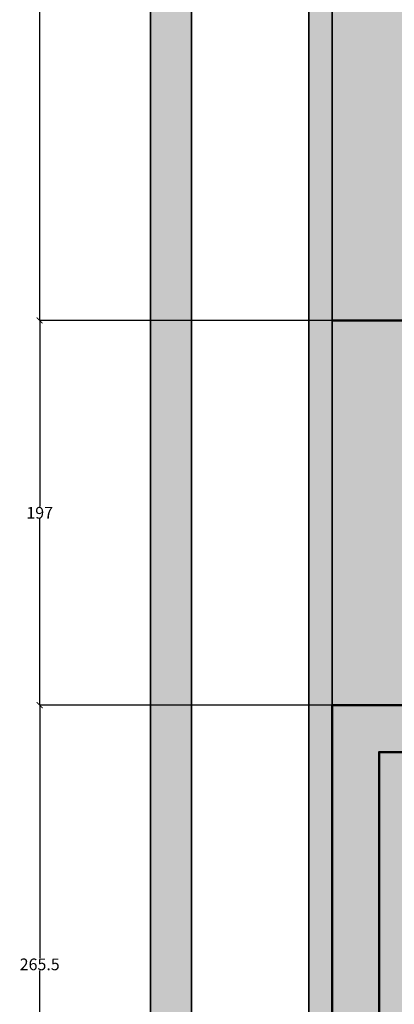
# Model space of a CAD drawing. Units: inches. Extents: x 925 to 2834, y 111 to 1355.
# Tile 2 of 25: x 925 to 1116, y 377 to 882. Entities that reach past the tile are written whole.
import ezdxf

# ---------------------------------------------------------------- set-up
doc = ezdxf.new("R2010")
doc.units = ezdxf.units.IN
doc.header["$MEASUREMENT"] = 0
for name, color, linetype, lineweight in [('A-ANNO-DIMS', 2, 'Continuous', 18), ('A-ANNO-TTLB', 7, 'Continuous', 35), ('A-FLOR-PATT', 252, 'Continuous', 13), ('A-WALL', 7, 'Continuous', 50)]:
    doc.layers.add(name, color=color, linetype=linetype, lineweight=lineweight)
doc.styles.get("Standard").update_dxf_attribs({"font": 'arial.ttf'})
doc.dimstyles.get("Standard").update_dxf_attribs({"dimtxt": 6, "dimasz": 3, "dimexe": 0.18, "dimexo": 0.0625, "dimgap": 0.09, "dimtad": 0, "dimtih": 1, "dimtoh": 1, "dimdec": 1, "dimzin": 0, "dimdsep": 46, "dimlunit": 3, "dimtxsty": 'Standard', "dimblk": 'ARCHTICK', "dimcen": 0.09, "dimadec": 0, "dimazin": 0, "dimtfac": 1, "dimtdec": 1, "dimtofl": 0, "dimtmove": 0, "dimatfit": 3, "dimfxl": 1, "dimtolj": 1, "dimtzin": 0, "dimarcsym": 0})

# ---------------------------------------------------------------- blocks, each defined once
blk = doc.blocks.new('_ArchTick')
at = {"color": 0, "linetype": 'ByBlock', "const_width": 0.15}
blk.add_lwpolyline([(-0.5, -0.5), (0.5, 0.5)], dxfattribs=at)
blk = doc.blocks.new('*D25')
at = {"layer": 'A-ANNO-DIMS', "color": 0, "lineweight": -2, "transparency": 16777216}
for p, q in [((1200.21, 727.53), (1200.21, 115.18)), ((1084.71, 265.03), (1084.71, 115.18)), ((1084.71, 115.36), (1132.51, 115.36)), ((1200.21, 115.36), (1152.42, 115.36))]:
    blk.add_line(p, q, dxfattribs=at)
at = {"layer": 'Defpoints', "color": 0, "transparency": 16777216}
for p in [(1200.21, 727.59), (1084.71, 265.09), (1200.21, 115.36)]:
    blk.add_point(p, dxfattribs=at)
at = {"layer": 'A-ANNO-DIMS', "color": 0, "lineweight": -2, "transparency": 16777216, "xscale": 3, "yscale": 3, "zscale": 3, "rotation": 180}
blk.add_blockref('_ArchTick', (1084.71, 115.36), dxfattribs=at)
at = {"layer": 'A-ANNO-DIMS', "color": 0, "lineweight": -2, "transparency": 16777216, "xscale": 3, "yscale": 3, "zscale": 3}
blk.add_blockref('_ArchTick', (1200.21, 115.36), dxfattribs=at)
at = {"layer": 'A-ANNO-DIMS', "color": 0, "transparency": 16777216, "insert": (1142.46, 115.36), "char_height": 6, "attachment_point": 5}
blk.add_mtext('\\A1;115.5', dxfattribs=at)
blk = doc.blocks.new('*D34')
at = {"layer": 'A-ANNO-DIMS', "color": 0, "lineweight": -2, "transparency": 16777216}
for p, q in [((1084.65, 530.59), (934.81, 530.59)), ((934.99, 530.59), (934.99, 400.99)), ((934.99, 265.09), (934.99, 394.69)), ((1084.65, 265.09), (934.81, 265.09))]:
    blk.add_line(p, q, dxfattribs=at)
at = {"layer": 'Defpoints', "color": 0, "transparency": 16777216}
for p in [(934.99, 530.59), (1084.71, 530.59), (1084.71, 265.09)]:
    blk.add_point(p, dxfattribs=at)
at = {"layer": 'A-ANNO-DIMS', "color": 0, "lineweight": -2, "transparency": 16777216, "xscale": 3, "yscale": 3, "zscale": 3}
for p, rotation in [((934.99, 530.59), 90), ((934.99, 265.09), 270)]:
    blk.add_blockref('_ArchTick', p, dxfattribs=dict(at, rotation=rotation))
at = {"layer": 'A-ANNO-DIMS', "color": 0, "transparency": 16777216, "insert": (934.99, 397.84), "char_height": 6, "attachment_point": 5}
blk.add_mtext('\\A1;265.5', dxfattribs=at)
blk = doc.blocks.new('*D35')
at = {"layer": 'A-ANNO-DIMS', "color": 0, "lineweight": -2, "transparency": 16777216}
for p, q in [((1084.65, 727.59), (934.81, 727.59)), ((934.99, 727.59), (934.99, 632.24)), ((934.99, 530.59), (934.99, 625.94)), ((1084.65, 530.59), (934.81, 530.59))]:
    blk.add_line(p, q, dxfattribs=at)
at = {"layer": 'Defpoints', "color": 0, "transparency": 16777216}
for p in [(934.99, 727.59), (1084.71, 727.59), (1084.71, 530.59)]:
    blk.add_point(p, dxfattribs=at)
at = {"layer": 'A-ANNO-DIMS', "color": 0, "lineweight": -2, "transparency": 16777216, "xscale": 3, "yscale": 3, "zscale": 3}
for p, rotation in [((934.99, 727.59), 90), ((934.99, 530.59), 270)]:
    blk.add_blockref('_ArchTick', p, dxfattribs=dict(at, rotation=rotation))
at = {"layer": 'A-ANNO-DIMS', "color": 0, "transparency": 16777216, "insert": (934.99, 629.09), "char_height": 6, "attachment_point": 5}
blk.add_mtext('\\A1;197', dxfattribs=at)
blk = doc.blocks.new('*D36')
at = {"layer": 'A-ANNO-DIMS', "color": 0, "lineweight": -2, "transparency": 16777216}
for p, q in [((1084.65, 1081.59), (934.81, 1081.59)), ((934.99, 1081.59), (934.99, 907.74)), ((934.99, 727.59), (934.99, 901.43)), ((1084.65, 727.59), (934.81, 727.59))]:
    blk.add_line(p, q, dxfattribs=at)
at = {"layer": 'Defpoints', "color": 0, "transparency": 16777216}
for p in [(934.99, 1081.59), (1084.71, 1081.59), (1084.71, 727.59)]:
    blk.add_point(p, dxfattribs=at)
at = {"layer": 'A-ANNO-DIMS', "color": 0, "lineweight": -2, "transparency": 16777216, "xscale": 3, "yscale": 3, "zscale": 3}
for p, rotation in [((934.99, 1081.59), 90), ((934.99, 727.59), 270)]:
    blk.add_blockref('_ArchTick', p, dxfattribs=dict(at, rotation=rotation))
at = {"layer": 'A-ANNO-DIMS', "color": 0, "transparency": 16777216, "insert": (934.99, 904.59), "char_height": 6, "attachment_point": 5}
blk.add_mtext('\\A1;354', dxfattribs=at)

msp = doc.modelspace()

# ---------------------------------------------------------------- hatches: boundary and pattern name
at = {"layer": 'A-FLOR-PATT', "transparency": 33554605}
h = msp.add_hatch(color=256, dxfattribs=at)
h.dxf.hatch_style = 1
h.paths.add_polyline_path([(1931.688, 1294.5638), (991.7375, 1294.5638), (991.7375, 172.1134), (1931.688, 172.1134)])
h.paths.add_polyline_path([(1910.7128, 1273.5886), (1910.7128, 193.0886), (1012.7128, 193.0886), (1012.7128, 1273.5886)], flags=16)
h.paths.add_polyline_path([(1850.7128, 1213.5886), (1850.7128, 253.0886), (1072.7128, 253.0886), (1072.7128, 1213.5886)], flags=0)
h.paths.add_polyline_path([(1838.7128, 1201.5886), (1838.7128, 265.0886), (1084.7128, 265.0886), (1084.7128, 530.5886), (1084.7128, 1201.5886)], flags=0)
h.paths.add_polyline_path([(1547.6758, 1155.7396), (1547.6758, 1119.115), (1513.0687, 1119.115), (1513.0687, 1155.7396)], flags=0)
h.paths.add_polyline_path([(1600.1067, 1154.9439), (1634.7139, 1154.9439), (1634.7139, 1119.115), (1600.1067, 1119.115)], flags=0)
h.paths.add_polyline_path([(1505.2502, 1144.5358), (1505.2502, 1119.115), (1470.643, 1119.115), (1470.643, 1144.5358)], flags=0)
h.paths.add_polyline_path([(1559.1357, 1141.0962), (1593.7428, 1141.0962), (1593.7428, 1119.115), (1559.1357, 1119.115)], flags=0)
h.paths.add_polyline_path([(1462.8966, 1154.9439), (1462.8966, 1119.115), (1428.2895, 1119.115), (1428.2895, 1154.9439)], flags=0)
h.paths.add_polyline_path([(1642.4603, 1144.5358), (1677.0675, 1144.5358), (1677.0675, 1119.115), (1642.4603, 1119.115)], flags=0)
h.paths.add_polyline_path([(1422.3508, 1141.0962), (1422.3508, 1119.115), (1387.7436, 1119.115), (1387.7436, 1141.0962)], flags=0)
h.paths.add_polyline_path([(1684.8859, 1155.7396), (1719.4931, 1155.7396), (1719.4931, 1119.115), (1684.8859, 1119.115)], flags=0)
h.paths.add_polyline_path([(1718.7128, 1081.5886), (1718.7128, 1050.1249), (1715.7128, 1050.1249), (1715.7128, 1026.1249), (1715.7128, 1002.1249), (1718.7128, 1002.1249), (1730.7128, 1002.1249), (1730.7128, 998.1249), (1730.7128, 990.1249), (1730.7128, 986.1249), (1718.7128, 986.1249), (1718.7128, 893.5886), (1715.3735, 893.5886), (1715.3735, 891.5886), (1713.3735, 891.5886, 0.41421356), (1677.3735, 855.5886), (1713.3735, 855.5886), (1713.3735, 853.5886), (1715.3735, 853.5886), (1715.3735, 851.5886), (1718.7128, 851.5886), (1718.7128, 821.5865), (1734.4655, 821.5865), (1734.3735, 819.5886, -0.41421356), (1712.4415, 793.5886), (1712.4415, 791.5886), (1718.7128, 791.5886), (1718.7128, 717.5886), (1718.7128, 669.5886), (1732.7128, 669.5886), (1732.7128, 665.5886), (1732.7128, 641.5886), (1732.7128, 634.5886), (1732.7128, 610.5886), (1732.7128, 603.5886), (1718.7128, 603.5886), (1718.7128, 385.0886), (1434.2128, 385.0886), (1434.2128, 530.5886), (1410.2128, 530.5886), (1408.2128, 530.5886), (1408.2128, 532.5886, 0.41421356), (1372.2128, 568.5886), (1372.2128, 532.5886), (1370.2128, 532.5886), (1370.2128, 530.5886), (1368.2128, 530.5886), (1282.2128, 530.5886), (1210.2128, 530.5886), (1200.2128, 530.5886), (1200.2128, 542.1915), (1183.2307, 542.1915), (1183.2307, 546.1915), (1200.2128, 546.1915), (1200.2128, 572.1915), (1183.2307, 572.1915), (1183.2307, 576.1915), (1200.2128, 576.1915), (1200.2128, 727.5886), (1210.2128, 727.5886), (1234.2128, 727.5886), (1259.7128, 727.5886), (1259.7128, 775.5886), (1259.7128, 799.5886), (1259.7128, 847.5886), (1259.7128, 993.5872), (1259.7128, 1065.5872), (1259.7128, 1071.5886), (1219.6318, 1071.5886), (1219.6318, 1081.5886), (1084.7128, 1081.5886), (1084.7128, 1119.115), (1256.8974, 1119.115), (1256.8974, 1154.9439), (1291.5046, 1154.9439), (1291.5046, 1119.115), (1256.8974, 1119.115), (1256.6723, 1081.5886), (1293.7128, 1081.5886), (1341.7128, 1081.5886), (1341.7128, 1093.5886), (1347.7128, 1093.5886), (1371.7128, 1093.5886), (1377.7128, 1093.5886), (1377.7128, 1081.5886), (1668.7128, 1081.5886), (1668.7128, 1117.5886), (1675.7128, 1117.5886), (1711.7128, 1117.5886), (1718.7128, 1117.5886)], flags=0)
h.paths.add_polyline_path([(1376.2838, 1155.7396), (1376.2838, 1119.115), (1341.6766, 1119.115), (1341.6766, 1155.7396)], flags=0)
h.paths.add_polyline_path([(1341.7128, 1076.0886), (1293.7128, 1076.0886), (1293.7128, 1071.5886), (1269.7128, 1071.5886), (1269.7128, 1065.5872), (1266.7128, 1065.5872), (1266.7128, 1029.5872), (1265.7128, 1029.5872), (1265.7128, 993.5872), (1269.7128, 993.5872), (1269.7128, 903.5886), (1269.7128, 893.5886), (1269.7128, 847.5886), (1265.2128, 847.5886), (1265.2128, 799.5886), (1269.7128, 799.5886), (1269.7128, 775.5886), (1265.2128, 775.5886), (1265.2128, 727.5886), (1269.7128, 727.5886), (1444.2128, 727.5886), (1444.2128, 717.5886), (1234.2128, 717.5886), (1234.2128, 722.0886), (1210.2128, 722.0886), (1210.2128, 717.5886), (1210.2128, 540.5886), (1210.2128, 536.0886), (1282.2128, 536.0886), (1282.2128, 535.0886), (1210.2128, 535.0886), (1210.2128, 540.5886), (1210.2128, 717.5886), (1210.2128, 723.0886), (1234.2128, 723.0886), (1234.2128, 717.5886), (1444.2128, 717.5886), (1444.2128, 727.5886), (1269.7128, 727.5886), (1264.2128, 727.5886), (1264.2128, 775.5886), (1269.7128, 775.5886), (1269.7128, 799.5886), (1264.2128, 799.5886), (1264.2128, 847.5886), (1269.7128, 847.5886), (1269.7128, 893.5886), (1269.7128, 903.5886), (1269.7128, 993.5872), (1264.7128, 993.5872), (1264.7128, 1029.5872), (1265.7128, 1029.5872), (1265.7128, 1065.5872), (1269.7128, 1065.5872), (1269.7128, 1071.5886), (1293.7128, 1071.5886), (1293.7128, 1077.0886), (1341.7128, 1077.0886)], flags=0)
h.paths.add_polyline_path([(1730.9529, 1141.0962), (1765.5601, 1141.0962), (1765.5601, 1119.115), (1730.9529, 1119.115)], flags=0)
h.paths.add_polyline_path([(1333.8582, 1144.5358), (1333.8582, 1119.115), (1299.251, 1119.115), (1299.251, 1144.5358)], flags=0)
h.paths.add_polyline_path([(1592.7128, 968.5886), (1596.0342, 968.5886), (1602.7128, 968.5886), (1708.7128, 968.5886), (1708.7128, 903.5886), (1602.7128, 903.5886), (1602.7128, 938.5886), (1592.7128, 938.5886), (1592.7128, 903.5886), (1451.7128, 903.5886), (1451.7128, 893.5886), (1511.7128, 893.5886), (1511.7128, 881.5886), (1515.2128, 881.5886), (1518.7128, 881.5886), (1518.7128, 893.5886), (1592.7128, 893.5886), (1592.7128, 799.5886), (1518.7128, 799.5886), (1518.7128, 857.5886), (1511.7128, 857.5886), (1511.7128, 799.5886), (1511.7128, 772.0886), (1521.7128, 772.0886), (1521.7128, 792.5886), (1592.7128, 792.5886), (1592.7128, 727.5886), (1521.7128, 727.5886), (1521.7128, 748.0886), (1511.7128, 748.0886), (1511.7128, 717.5886), (1708.7128, 717.5886), (1714.2128, 717.5886), (1714.2128, 669.5886), (1708.7128, 669.5886), (1708.7128, 641.5886), (1492.2128, 641.5886), (1492.2128, 631.5886), (1621.2128, 631.5886), (1621.2128, 443.0886), (1625.7128, 443.0886), (1625.7128, 503.0886), (1625.7128, 507.5886), (1625.7128, 631.5886), (1708.7128, 631.5886), (1708.7128, 507.5886), (1655.7128, 507.5886), (1655.7128, 503.0886), (1708.7128, 503.0886), (1708.7128, 395.0886), (1625.7128, 395.0886), (1625.7128, 419.0886), (1621.2128, 419.0886), (1621.2128, 395.0886), (1482.2128, 395.0886), (1482.2128, 385.0886), (1434.2128, 385.0886), (1434.2128, 433.0886), (1444.2128, 433.0886), (1444.2128, 631.5886), (1450.2128, 631.5886), (1450.2128, 634.91), (1452.2128, 634.91), (1452.2128, 669.5886), (1454.2128, 669.5886, -0.40021217), (1490.1712, 635.3173), (1492.2128, 635.3173), (1492.2128, 641.5886), (1564.7128, 641.5886), (1564.7128, 677.5886), (1672.7128, 677.5886), (1672.7128, 681.5886), (1564.7128, 681.5886), (1564.7128, 717.5886), (1511.7128, 717.5886), (1511.7128, 748.0886), (1511.7128, 772.0886), (1511.7128, 799.5886), (1511.7128, 857.5886), (1511.8913, 857.5886), (1511.8913, 859.5886), (1515.6201, 859.5886, 0.41421356), (1537.552, 879.5886), (1513.552, 879.5886), (1511.8913, 879.5886), (1511.8913, 881.5886), (1511.7128, 881.5886), (1511.7128, 893.5886), (1451.7128, 893.5886), (1451.7128, 903.5886), (1592.7128, 903.5886), (1592.7128, 938.5886), (1592.7128, 940.5886), (1596.4415, 940.5886, 0.41421356), (1618.3735, 966.5886), (1594.3735, 966.5886), (1592.7128, 966.5886)], flags=0)
h.paths.add_polyline_path([(1377.7128, 903.5886), (1377.7128, 893.5886), (1305.7128, 893.5886), (1305.7128, 903.5886)], flags=0)
h.paths.add_polyline_path([(1708.7128, 821.5886), (1712.0342, 821.5886), (1712.0342, 819.5886), (1710.3735, 819.5886), (1708.7128, 819.5886)], flags=0)
h.paths.add_polyline_path([(1576.7128, 695.1992), (1575.5896, 693.6649), (1575.9687, 694.6994), (1575.4438, 695.1992), (1575.9687, 695.699), (1575.5896, 696.7335)], flags=0)
h.paths.add_polyline_path([(1565.9817, 662.3134), (1565.4568, 661.8136), (1565.8359, 660.7791), (1564.7128, 662.3134), (1565.8359, 663.8477), (1565.4568, 662.8132)], flags=0)
h.paths.add_polyline_path([(1444.2128, 433.0886), (1444.2128, 395.0886), (1482.2128, 395.0886), (1482.2128, 389.0886), (1438.2128, 389.0886), (1438.2128, 391.8608), (1438.2128, 433.0886)], flags=0)
h.paths.add_polyline_path([(1410.2128, 506.5886), (1410.2128, 289.0886), (1108.7128, 289.0886), (1108.7128, 506.5886)], flags=0)
h.paths.add_polyline_path([(1612.3153, 838.3016), (1680.4151, 838.3016), (1680.4151, 851.3131), (1612.3153, 851.3131)], flags=8)
h.paths.add_polyline_path([(1208.3174, 395.0436), (1282.1017, 395.0436), (1282.1017, 408.0552), (1208.3174, 408.0552)], flags=8)
h.paths.add_polyline_path([(1291.8049, 598.7427), (1369.8017, 598.7427), (1369.8017, 611.7542), (1291.8049, 611.7542)], flags=8)
h.paths.add_polyline_path([(1119.679, 917.3022), (1191.0817, 917.3022), (1191.0817, 930.3137), (1119.679, 930.3137)], flags=8)
h.paths.add_polyline_path([(1332.2261, 815.9808), (1410.2258, 815.9808), (1410.2258, 829.001), (1332.2261, 829.001)], flags=8)
h.paths.add_polyline_path([(1390.9013, 955.8158), (1475.4981, 955.8158), (1475.4981, 968.8273), (1390.9013, 968.8273)], flags=8)
h.paths.add_polyline_path([(1620.3436, 998.9325), (1688.4434, 998.9325), (1688.4434, 1011.944), (1620.3436, 1011.944)], flags=8)
h.paths.add_polyline_path([(1620.3436, 914.1039), (1691.7405, 914.1039), (1691.7405, 927.1155), (1620.3436, 927.1155)], flags=8)
h.paths.add_polyline_path([(1521.4542, 816.005), (1589.5569, 816.005), (1589.5569, 829.0253), (1521.4542, 829.0253)], flags=8)
h.paths.add_polyline_path([(1528.524, 740.3497), (1602.3082, 740.3497), (1602.3082, 753.3613), (1528.524, 753.3613)], flags=8)
h.paths.add_polyline_path([(1627.6094, 762.6128), (1702.3091, 762.6128), (1702.3091, 775.6244), (1627.6094, 775.6244)], flags=8)
h.paths.add_polyline_path([(1610.5442, 657.2751), (1684.3284, 657.2751), (1684.3284, 670.2867), (1610.5442, 670.2867)], flags=8)
h.paths.add_polyline_path([(1636.6983, 519.472), (1711.3981, 519.472), (1711.3981, 532.4835), (1636.6983, 532.4835)], flags=8)
h.paths.add_polyline_path([(1616.8577, 424.8539), (1694.8545, 424.8539), (1694.8545, 437.8654), (1616.8577, 437.8654)], flags=8)
h.paths.add_polyline_path([(1506.1456, 460.8838), (1579.9299, 460.8838), (1579.9299, 473.8953), (1506.1456, 473.8953)], flags=8)
h.paths.add_polyline_path([(1624.6119, 784.6011), (1696.9185, 784.6011), (1696.9185, 797.7864), (1624.6119, 797.7864)], flags=8)
h.paths.add_polyline_path([(1606.3732, 854.2194), (1683.3039, 854.2194), (1683.3039, 867.4048), (1606.3732, 867.4048)], flags=8)
h.paths.add_polyline_path([(1127.8008, 940.3581), (1165.1637, 940.3581), (1165.1637, 953.5348), (1127.8008, 953.5348)], flags=8)
h.paths.add_polyline_path([(1620.8657, 1019.4968), (1677.3447, 1019.4968), (1677.3447, 1032.6735), (1620.8657, 1032.6735)], flags=8)
h.paths.add_polyline_path([(1620.8643, 930.1821), (1703.0564, 930.1821), (1703.0564, 943.3675), (1620.8643, 943.3675)], flags=8)
h.paths.add_polyline_path([(1324.5702, 836.8338), (1408.0892, 836.8338), (1408.0892, 850.0191), (1324.5702, 850.0191)], flags=8)
h.paths.add_polyline_path([(1281.6584, 622.8885), (1383.6213, 622.8885), (1383.6213, 636.0739), (1281.6584, 636.0739)], flags=8)
h.paths.add_polyline_path([(1210.6721, 416.7893), (1269.1299, 416.7893), (1269.1299, 429.9747), (1210.6721, 429.9747)], flags=8)
h.paths.add_polyline_path([(1507.8264, 477.4836), (1586.7329, 477.4836), (1586.7329, 490.669), (1507.8264, 490.669)], flags=8)
h.paths.add_polyline_path([(1643.6238, 443.8135), (1696.6696, 443.8135), (1696.6696, 456.5643), (1643.6238, 456.5643)], flags=8)
h.paths.add_polyline_path([(1647.2466, 540.5638), (1693.1825, 540.5638), (1693.1825, 553.7491), (1647.2466, 553.7491)], flags=8)
h.paths.add_polyline_path([(1626.0633, 668.5064), (1673.3174, 668.5064), (1673.3174, 681.6831), (1626.0633, 681.6831)], flags=8)
h.paths.add_polyline_path([(1538.2915, 830.7872), (1567.5942, 830.7872), (1567.5942, 843.5293), (1538.2915, 843.5293)], flags=8)
h.paths.add_polyline_path([(1530.9338, 754.0477), (1559.576, 754.0477), (1559.576, 766.7898), (1530.9338, 766.7898)], flags=8)
h.paths.add_polyline_path([(1351.2461, 979.2309), (1513.8919, 979.2309), (1513.8919, 992.4076), (1351.2461, 992.4076)], flags=8)
at = {"layer": 'A-FLOR-PATT'}
h = msp.add_hatch(color=256, dxfattribs=at)
h.dxf.hatch_style = 1
h.paths.add_polyline_path([(1850.7128, 1213.5886), (1072.7128, 1213.5886), (1072.7128, 253.0886), (1850.7128, 253.0886)])
h.paths.add_polyline_path([(1084.7128, 1201.5886), (1838.7128, 1201.5886), (1838.7128, 265.0886), (1084.7128, 265.0886)], flags=16)
h.paths.add_polyline_path([(1183.2307, 576.1915), (1200.2128, 576.1915), (1200.2128, 727.5886), (1210.2128, 727.5886), (1234.2128, 727.5886), (1259.7128, 727.5886), (1259.7128, 775.5886), (1259.7128, 799.5886), (1259.7128, 847.5886), (1259.7128, 993.5872), (1259.7128, 1065.5872), (1259.7128, 1071.5886), (1219.6318, 1071.5886), (1219.6318, 1081.5886), (1293.7128, 1081.5886), (1341.7128, 1081.5886), (1341.7128, 1093.5886), (1347.7128, 1093.5886), (1347.7128, 1081.5886), (1371.7128, 1081.5886), (1371.7128, 1093.5886), (1377.7128, 1093.5886), (1377.7128, 1081.5886), (1668.7128, 1081.5886), (1668.7128, 1117.5886), (1675.7128, 1117.5886), (1675.7128, 1081.5886), (1711.7128, 1081.5886), (1711.7128, 1117.5886), (1718.7128, 1117.5886), (1718.7128, 1081.5886), (1718.7128, 1050.1249), (1715.7128, 1050.1249), (1715.7128, 1026.1249), (1715.7128, 1002.1249), (1718.7128, 1002.1249), (1730.7128, 1002.1249), (1730.7128, 998.1249), (1730.7128, 990.1249), (1730.7128, 986.1249), (1718.7128, 986.1249), (1718.7128, 893.5886), (1715.3735, 893.5886), (1715.3735, 891.5886), (1713.3735, 891.5886, 0.41421356), (1677.3735, 855.5886), (1713.3735, 855.5886), (1713.3735, 853.5886), (1715.3735, 853.5886), (1715.3735, 851.5886), (1718.7128, 851.5886), (1718.7128, 821.5865), (1734.4655, 821.5865), (1734.3735, 819.5886, -0.41421356), (1712.4415, 793.5886), (1712.4415, 791.5886), (1718.7128, 791.5886), (1718.7128, 717.5886), (1718.7128, 669.5886), (1732.7128, 669.5886), (1732.7128, 665.5886), (1732.7128, 641.5886), (1732.7128, 634.5886), (1732.7128, 610.5886), (1732.7128, 603.5886), (1718.7128, 603.5886), (1718.7128, 385.0886), (1434.2128, 385.0886), (1434.2128, 433.0886), (1434.2128, 530.5886), (1410.2128, 530.5886), (1408.2128, 530.5886), (1408.2128, 532.5886, 0.41421356), (1372.2128, 568.5886), (1372.2128, 532.5886), (1370.2128, 532.5886), (1370.2128, 530.5886), (1368.2128, 530.5886), (1282.2128, 530.5886), (1210.2128, 530.5886), (1200.2128, 530.5886), (1200.2128, 542.1915), (1183.2307, 542.1915), (1183.2307, 546.1915), (1200.2128, 546.1915), (1200.2128, 572.1915), (1183.2307, 572.1915)], flags=0)
h.paths.add_polyline_path([(1210.2128, 717.5886), (1210.2128, 723.0886), (1234.2128, 723.0886), (1234.2128, 717.5886), (1444.2128, 717.5886), (1444.2128, 727.5886), (1269.7128, 727.5886), (1264.2128, 727.5886), (1264.2128, 775.5886), (1269.7128, 775.5886), (1269.7128, 799.5886), (1264.2128, 799.5886), (1264.2128, 847.5886), (1269.7128, 847.5886), (1269.7128, 893.5886), (1269.7128, 903.5886), (1269.7128, 993.5872), (1264.7128, 993.5872), (1264.7128, 1029.5872), (1265.7128, 1029.5872), (1265.7128, 1065.5872), (1269.7128, 1065.5872), (1269.7128, 1071.5886), (1293.7128, 1071.5886), (1293.7128, 1077.0886), (1341.7128, 1077.0886), (1341.7128, 1076.0886), (1293.7128, 1076.0886), (1293.7128, 1071.5886), (1269.7128, 1071.5886), (1269.7128, 1065.5872), (1266.7128, 1065.5872), (1266.7128, 1029.5872), (1265.7128, 1029.5872), (1265.7128, 993.5872), (1269.7128, 993.5872), (1269.7128, 903.5886), (1269.7128, 893.5886), (1269.7128, 847.5886), (1265.2128, 847.5886), (1265.2128, 799.5886), (1269.7128, 799.5886), (1269.7128, 775.5886), (1265.2128, 775.5886), (1265.2128, 727.5886), (1269.7128, 727.5886), (1444.2128, 727.5886), (1444.2128, 717.5886), (1234.2128, 717.5886), (1234.2128, 722.0886), (1210.2128, 722.0886), (1210.2128, 717.5886), (1210.2128, 540.5886), (1210.2128, 536.0886), (1282.2128, 536.0886), (1282.2128, 535.0886), (1210.2128, 535.0886), (1210.2128, 540.5886)], flags=0)
h.paths.add_polyline_path([(1450.2128, 634.91), (1452.2128, 634.91), (1452.2128, 669.5886), (1454.2128, 669.5886, -0.40021217), (1490.1712, 635.3173), (1492.2128, 635.3173), (1492.2128, 641.5886), (1564.7128, 641.5886), (1564.7128, 677.5886), (1672.7128, 677.5886), (1672.7128, 681.5886), (1564.7128, 681.5886), (1564.7128, 717.5886), (1511.7128, 717.5886), (1511.7128, 748.0886), (1511.7128, 772.0886), (1511.7128, 799.5886), (1511.7128, 857.5886), (1511.8913, 857.5886), (1511.8913, 859.5886), (1515.6201, 859.5886, 0.41421356), (1537.552, 879.5886), (1513.552, 879.5886), (1511.8913, 879.5886), (1511.8913, 881.5886), (1511.7128, 881.5886), (1511.7128, 893.5886), (1451.7128, 893.5886), (1451.7128, 903.5886), (1592.7128, 903.5886), (1592.7128, 938.5886), (1592.7128, 940.5886), (1596.4415, 940.5886, 0.41421356), (1618.3735, 966.5886), (1594.3735, 966.5886), (1592.7128, 966.5886), (1592.7128, 968.5886), (1596.0342, 968.5886), (1602.7128, 968.5886), (1708.7128, 968.5886), (1708.7128, 903.5886), (1602.7128, 903.5886), (1602.7128, 938.5886), (1592.7128, 938.5886), (1592.7128, 903.5886), (1451.7128, 903.5886), (1451.7128, 893.5886), (1511.7128, 893.5886), (1511.7128, 881.5886), (1518.7128, 881.5886), (1518.7128, 893.5886), (1592.7128, 893.5886), (1592.7128, 799.5886), (1518.7128, 799.5886), (1518.7128, 857.5886), (1511.7128, 857.5886), (1511.7128, 799.5886), (1511.7128, 772.0886), (1521.7128, 772.0886), (1521.7128, 792.5886), (1592.7128, 792.5886), (1592.7128, 727.5886), (1521.7128, 727.5886), (1521.7128, 748.0886), (1511.7128, 748.0886), (1511.7128, 717.5886), (1708.7128, 717.5886), (1714.2128, 717.5886), (1714.2128, 669.5886), (1708.7128, 669.5886), (1708.7128, 641.5886), (1492.2128, 641.5886), (1492.2128, 631.5886), (1621.2128, 631.5886), (1621.2128, 443.0886), (1625.7128, 443.0886), (1625.7128, 503.0886), (1625.7128, 507.5886), (1625.7128, 631.5886), (1708.7128, 631.5886), (1708.7128, 507.5886), (1655.7128, 507.5886), (1655.7128, 503.0886), (1708.7128, 503.0886), (1708.7128, 395.0886), (1625.7128, 395.0886), (1625.7128, 419.0886), (1621.2128, 419.0886), (1621.2128, 395.0886), (1482.2128, 395.0886), (1482.2128, 389.0886), (1438.2128, 389.0886), (1438.2128, 391.8608), (1438.2128, 433.0886), (1444.2128, 433.0886), (1444.2128, 631.5886), (1450.2128, 631.5886)], flags=0)
h.paths.add_polyline_path([(1444.2128, 433.0886), (1444.2128, 395.0886), (1482.2128, 395.0886), (1482.2128, 391.0886), (1440.2128, 391.0886), (1440.2128, 391.8608), (1440.2128, 433.0886)], flags=0)
h.paths.add_polyline_path([(1305.7128, 893.5886), (1305.7128, 903.5886), (1377.7128, 903.5886), (1377.7128, 893.5886)], flags=0)
h.paths.add_polyline_path([(1564.7128, 662.3134), (1565.8359, 663.8477), (1565.4568, 662.8132), (1565.9817, 662.3134), (1565.4568, 661.8136), (1565.8359, 660.7791)], flags=0)
h.paths.add_polyline_path([(1575.4438, 695.1992), (1575.9687, 695.699), (1575.5896, 696.7335), (1576.7128, 695.1992), (1575.5896, 693.6649), (1575.9687, 694.6994)], flags=0)
h.paths.add_polyline_path([(1708.7128, 821.5886), (1712.0342, 821.5886), (1712.0342, 819.5886), (1710.3735, 819.5886), (1708.7128, 819.5886)], flags=0)
at = {"layer": 'A-FLOR-PATT', "transparency": 33554574}
h = msp.add_hatch(color=256, dxfattribs=at)
h.dxf.hatch_style = 1
h.paths.add_polyline_path([(1259.7128, 993.5872), (1259.7128, 1065.5872), (1259.7128, 1071.5886), (1219.6318, 1071.5886), (1219.6318, 1081.5886), (1084.7128, 1081.5886), (1084.7128, 727.5886), (1200.2128, 727.5886), (1210.2128, 727.5886), (1234.2128, 727.5886), (1259.7128, 727.5886), (1259.7128, 775.5886), (1259.7128, 799.5886), (1259.7128, 847.5886)])
at = {"layer": 'A-FLOR-PATT', "transparency": 33554605}
h = msp.add_hatch(color=256, dxfattribs=at)
h.dxf.hatch_style = 1
h.paths.add_polyline_path([(1200.2128, 727.5886), (1084.7128, 727.5886), (1084.7128, 530.5886), (1200.2128, 530.5886), (1200.2128, 542.1915), (1183.2307, 542.1915), (1183.2307, 546.1915), (1200.2128, 546.1915), (1200.2128, 572.1915), (1183.2307, 572.1915), (1183.2307, 576.1915), (1200.2128, 576.1915)])
h.paths.add_polyline_path([(1612.3153, 838.3016), (1680.4151, 838.3016), (1680.4151, 851.3131), (1612.3153, 851.3131)], flags=9)
h.paths.add_polyline_path([(1291.8049, 598.7427), (1369.8017, 598.7427), (1369.8017, 611.7542), (1291.8049, 611.7542)], flags=9)
h.paths.add_polyline_path([(1119.679, 917.3022), (1191.0817, 917.3022), (1191.0817, 930.3137), (1119.679, 930.3137)], flags=9)
h.paths.add_polyline_path([(1332.2261, 815.9808), (1410.2258, 815.9808), (1410.2258, 829.001), (1332.2261, 829.001)], flags=9)
h.paths.add_polyline_path([(1390.9013, 955.8158), (1475.4981, 955.8158), (1475.4981, 968.8273), (1390.9013, 968.8273)], flags=9)
h.paths.add_polyline_path([(1620.3436, 998.9325), (1688.4434, 998.9325), (1688.4434, 1011.944), (1620.3436, 1011.944)], flags=9)
h.paths.add_polyline_path([(1620.3436, 914.1039), (1691.7405, 914.1039), (1691.7405, 927.1155), (1620.3436, 927.1155)], flags=9)
h.paths.add_polyline_path([(1521.4542, 816.005), (1589.5569, 816.005), (1589.5569, 829.0253), (1521.4542, 829.0253)], flags=9)
h.paths.add_polyline_path([(1522.4337, 740.3497), (1596.218, 740.3497), (1596.218, 753.3613), (1522.4337, 753.3613)], flags=9)
h.paths.add_polyline_path([(1606.3732, 854.2194), (1683.3039, 854.2194), (1683.3039, 867.4048), (1606.3732, 867.4048)], flags=9)
h.paths.add_polyline_path([(1127.8008, 940.3581), (1165.1637, 940.3581), (1165.1637, 953.5348), (1127.8008, 953.5348)], flags=9)
h.paths.add_polyline_path([(1620.8657, 1019.4968), (1677.3447, 1019.4968), (1677.3447, 1032.6735), (1620.8657, 1032.6735)], flags=9)
h.paths.add_polyline_path([(1620.8643, 930.1821), (1703.0564, 930.1821), (1703.0564, 943.3675), (1620.8643, 943.3675)], flags=9)
h.paths.add_polyline_path([(1324.5702, 836.8338), (1408.0892, 836.8338), (1408.0892, 850.0191), (1324.5702, 850.0191)], flags=9)
h.paths.add_polyline_path([(1281.6584, 622.8885), (1383.6213, 622.8885), (1383.6213, 636.0739), (1281.6584, 636.0739)], flags=9)
h.paths.add_polyline_path([(1626.0633, 668.5064), (1673.3174, 668.5064), (1673.3174, 681.6831), (1626.0633, 681.6831)], flags=9)
h.paths.add_polyline_path([(1538.2915, 830.7872), (1567.5942, 830.7872), (1567.5942, 843.5293), (1538.2915, 843.5293)], flags=9)
h.paths.add_polyline_path([(1351.2461, 979.2309), (1513.8919, 979.2309), (1513.8919, 992.4076), (1351.2461, 992.4076)], flags=9)
at = {"layer": 'A-FLOR-PATT', "transparency": 33554498}
h = msp.add_hatch(color=256, dxfattribs=at)
h.dxf.hatch_style = 1
h.paths.add_polyline_path([(1434.2128, 530.5886), (1084.7128, 530.5886), (1084.7128, 265.0886), (1434.2128, 265.0886)])
h.paths.add_polyline_path([(1410.2128, 506.5886), (1410.2128, 289.0886), (1108.7128, 289.0886), (1108.7128, 506.5886)], flags=16)
h.paths.add_polyline_path([(1410.2128, 506.5886), (1108.7128, 506.5886), (1108.7128, 289.0886), (1410.2128, 289.0886)], flags=16)

# ---------------------------------------------------------------- linework, layer by layer
at = {"layer": 'A-ANNO-TTLB'}
for points in [[(991.7375, 172.1134), (1931.688, 172.1134), (1931.688, 1294.5638), (991.7375, 1294.5638)], [(1012.7128, 193.0886), (1910.7128, 193.0886), (1910.7128, 1273.5886), (1012.7128, 1273.5886)], [(1072.7128, 253.0886), (1850.7128, 253.0886), (1850.7128, 1213.5886), (1072.7128, 1213.5886)], [(1084.7128, 265.0886), (1838.7128, 265.0886), (1838.7128, 1201.5886), (1084.7128, 1201.5886)]]:
    msp.add_lwpolyline(points, close=True, dxfattribs=at)
at = {"layer": 'A-WALL'}
for p, q in [((1200.2128, 727.5886), (1084.7128, 727.5886)), ((1084.7128, 530.5886), (1084.7128, 265.0886))]:
    msp.add_line(p, q, dxfattribs=at)
for points in [[(1434.2128, 530.5886), (1084.7128, 530.5886), (1084.7128, 265.0886), (1434.2128, 265.0886)], [(1410.2128, 506.5886), (1108.7128, 506.5886), (1108.7128, 289.0886), (1410.2128, 289.0886)]]:
    msp.add_lwpolyline(points, close=True, dxfattribs=at)

# ---------------------------------------------------------------- dimensions: what is measured, and where the dimension line sits
at = {"layer": 'A-ANNO-DIMS'}
for base, p1, p2, override, picture, middle in [((934.9875, 1081.5886), (1084.7128, 727.5886), (1084.7128, 1081.5886), {"dimdec": 0, "dimlfac": 1, "dimrnd": 0, "dimzin": 0, "dimdsep": 46, "dimlunit": 2}, '*D36', (934.9875, 904.5886)), ((934.9875, 727.5886), (1084.7128, 530.5886), (1084.7128, 727.5886), {"dimdec": 0, "dimlfac": 1, "dimrnd": 0, "dimzin": 0, "dimdsep": 46, "dimlunit": 2}, '*D35', (934.9875, 629.0886)), ((934.9875, 530.5886), (1084.7128, 265.0886), (1084.7128, 530.5886), {"dimdec": 1, "dimlfac": 1, "dimrnd": 0, "dimzin": 0, "dimdsep": 46, "dimlunit": 2}, '*D34', (934.9875, 397.8386))]:
    dim = msp.add_linear_dim(base=base, p1=p1, p2=p2, angle=90, dimstyle='Standard', override=override, dxfattribs=at)
    dim.commit()
    dim.dimension.update_dxf_attribs({"geometry": picture, "text_midpoint": middle})
dim = msp.add_linear_dim(base=(1200.2128, 115.3634), p1=(1084.7128, 265.0886), p2=(1200.2128, 727.5886), dimstyle='Standard', override={"dimdec": 1, "dimlfac": 1, "dimrnd": 0, "dimzin": 0, "dimdsep": 46, "dimlunit": 2}, dxfattribs=at)
dim.commit()
dim.dimension.update_dxf_attribs({"geometry": '*D25', "text_midpoint": (1142.4628, 115.3634)})

doc.saveas('drawing.dxf')
